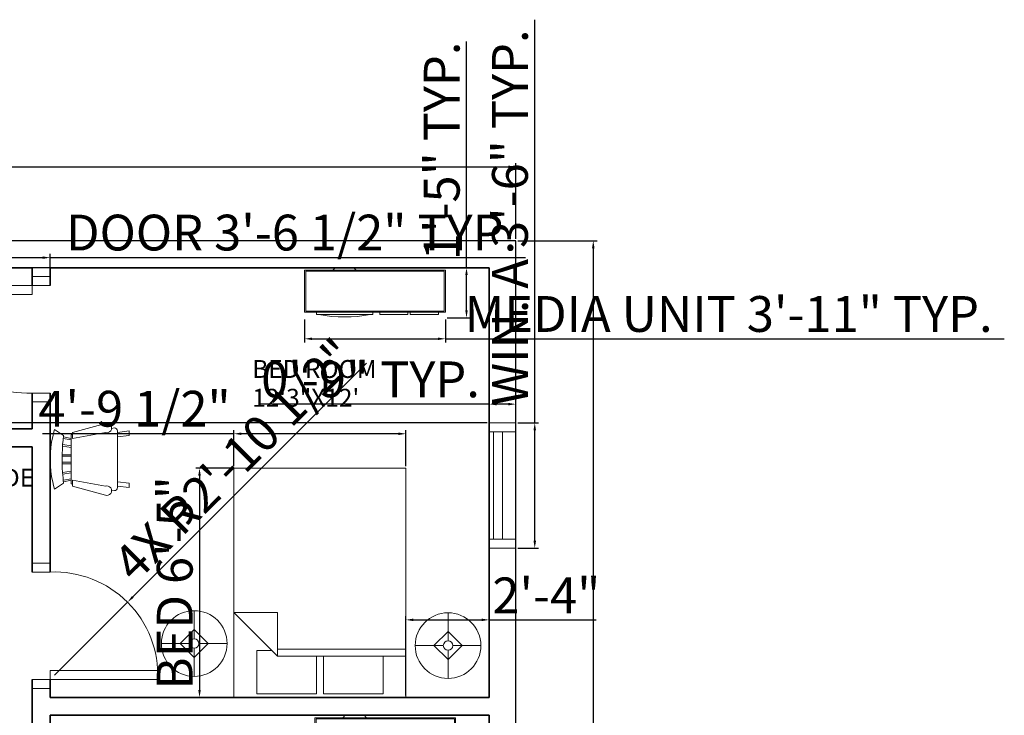
# Model space of a CAD drawing. Units: inches. Extents: x 2021 to 2692, y 429 to 1061.
# Tile 5 of 5: x 2362 to 2692, y 828 to 1061. Entities that reach past the tile are written whole.
import ezdxf

# ---------------------------------------------------------------- set-up
doc = ezdxf.new("R2010")
doc.units = ezdxf.units.IN
for name, color, linetype, lineweight in [('A-ANNO-DIMS', 2, 'Continuous', 18), ('A-AREA-IDEN', 7, 'Continuous', 18), ('A-DOOR', 4, 'Continuous', 18), ('A-FURN', 8, 'Continuous', 13), ('A-GLAZ', 4, 'Continuous', 18), ('A-WALL', 7, 'Continuous', 35), ('C-PROP', 3, 'Continuous', 25)]:
    doc.layers.add(name, color=color, linetype=linetype, lineweight=lineweight)
doc.styles.get("Standard").update_dxf_attribs({"font": 'arial.ttf'})
doc.dimstyles.new('ISO-25', dxfattribs={"dimtxt": 12, "dimasz": 2.5, "dimexe": 1.25, "dimexo": 0.625, "dimtad": 1, "dimdec": 0, "dimlunit": 3, "dimtxsty": 'Standard', "dimcen": 2.5, "dimadec": 0, "dimazin": 0, "dimtfac": 1, "dimtdec": 0, "dimtmove": 0, "dimatfit": 3, "dimfxl": 1, "dimarcsym": 0})

# ---------------------------------------------------------------- blocks, each defined once
blk = doc.blocks.new('Bed - Queen')
for p, q in [((0, -80.00003), (0, 0)), ((0, 0), (59.99999, 0)), ((59.99999, 0), (59.99999, -80.00003)), ((7.99999, -1.2), (28.79998, -1.2)), ((7.99999, -14.4), (7.99999, -1.2)), ((28.79998, -1.2), (28.79998, -14.4)), ((31.19999, -1.2), (51.99999, -1.2)), ((31.19999, -14.4), (31.19999, -1.2)), ((51.99999, -1.2), (51.99999, -16.4)), ((0, -14.4), (44.8, -14.4)), ((44.8, -16.8), (0, -16.8)), ((59.99999, -29.6), (44.8, -14.4)), ((44.8, -14.4), (44.8, -29.6)), ((51.99999, -16.4), (46.79936, -16.4)), ((44.8, -29.6), (59.99999, -29.6)), ((59.99999, -80.00003), (0, -80.00003))]:
    blk.add_line(p, q)
blk = doc.blocks.new('Entertainment Center')
for p, q in [((-4, 0), (-5, -1)), ((4, 0), (-4, 0)), ((5, -1), (4, 0)), ((-17, -19), (-17, -1)), ((-17, -1), (43, -1)), ((-16.5, -18.5), (-16.5, -1.5)), ((-16.5, -1.5), (42.5, -1.5)), ((42.5, -1.5), (42.5, -18.5)), ((43, -1), (43, -19)), ((43, -19), (-17, -19)), ((42.5, -18.5), (-16.5, -18.5)), ((-12, -20), (-12, -19)), ((12, -20), (-12, -20)), ((12, -19), (12, -20)), ((15, -20), (15, -19)), ((27, -20), (15, -20)), ((27, -19), (27, -20)), ((28, -20), (28, -19)), ((40, -20), (28, -20)), ((40, -19), (40, -20))]:
    blk.add_line(p, q)
blk.add_arc((0, 40), 61, 259.6111, 280.3889)
blk = doc.blocks.new('Chair - Rocking')
for p, q in [((-8, -4.5), (-10, -1.5)), ((8, -4.5), (10, -1.5)), ((-7.5, -4.5), (-7, -7)), ((-6.5, -7), (-7.02225, -4.43)), ((-4.5, -7), (-4.96674, -4.19951)), ((-4, -7), (-4.40532, -4.16272)), ((-1.5, -4.05012), (-1.5, -7)), ((-1, -7), (-1, -4.05012)), ((1, -7), (1, -4.04655)), ((1.5, -4.05012), (1.5, -7)), ((4, -7), (4.40187, -4.18694)), ((4.5, -7), (4.96761, -4.19437)), ((6.5, -7), (7, -4.4057)), ((7.5, -4.5), (7, -7)), ((-9, -7.5), (-12, -18.49999)), ((-7, -7.5), (-9, -7.5)), ((-9, -18.49999), (-7, -7.5)), ((-8.23428, -6.99939), (-8.3093, -7.47958)), ((-8.23041, -7), (8.23915, -7)), ((7, -7.5), (9, -7.5)), ((9, -18.49999), (7, -7.5)), ((8.31071, -7.48854), (8.23449, -7.00073)), ((9, -7.5), (12, -18.49999)), ((-10.36644, -20.64523), (-10.5, -21.49999)), ((-9, -22.49999), (-9.5, -26.49999)), ((0, -22.49999), (-9.5, -22.49999)), ((-8, -26.49999), (-7.5, -22.49999)), ((0, -22.49999), (9.5, -22.49999)), ((8, -26.49999), (7.5, -22.49999)), ((9, -22.49999), (9.5, -26.49999)), ((10.5, -21.49999), (10.3575, -20.58798)), ((-9.5, -26.49999), (-8, -26.49999)), ((9.5, -26.49999), (8, -26.49999))]:
    blk.add_line(p, q)
for centre, radius, start, end in [((0, -34.08333), 34.08333, 72.93847, 107.0615), ((0, -68.25004), 64.25, 93.92211, 97.15267), ((0, -68.25004), 64.25, 82.84733, 93.92211), ((-10.5, -18.99999), 1.58114, 161.5651, 18.43495), ((10.5, -18.99999), 1.58114, 161.5651, 18.43495), ((-9.5, -21.49999), 1, 180, 270), ((9.5, -21.49999), 1, 270, 0)]:
    blk.add_arc(centre, radius, start, end)
blk = doc.blocks.new('Lamp - Table')
for p, q in [((0, 7), (0, 1)), ((0, 3), (-3, 0)), ((3, 0), (0, 3)), ((-1, 0), (-7, 0)), ((-3, 0), (0, -3)), ((0, -3), (3, 0)), ((1, 0), (7, 0)), ((0, -1), (0, -7))]:
    blk.add_line(p, q)
for radius in [7, 1]:
    blk.add_circle((0, 0), radius)
blk = doc.blocks.new('*D15')
at = {"layer": 'A-ANNO-DIMS', "color": 0, "lineweight": -2, "transparency": 16777216}
for p, q in [((2168.11, 987.59), (2168.11, 1013.02)), ((2528.11, 987.59), (2528.11, 1013.02)), ((2170.61, 1011.77), (2525.61, 1011.77))]:
    blk.add_line(p, q, dxfattribs=at)
at = {"layer": 'A-ANNO-DIMS', "color": 0, "transparency": 16777216}
for points in [[(2170.61, 1012.18), (2170.61, 1011.35), (2168.11, 1011.77)], [(2525.61, 1012.18), (2525.61, 1011.35), (2528.11, 1011.77)]]:
    blk.add_solid(points, dxfattribs=at)
at = {"layer": 'Defpoints', "color": 0, "transparency": 16777216}
for p in [(2528.11, 1011.77), (2168.11, 986.96), (2528.11, 986.96)]:
    blk.add_point(p, dxfattribs=at)
at = {"layer": 'A-ANNO-DIMS', "color": 0, "transparency": 16777216, "insert": (2348.11, 1018.52), "char_height": 12, "attachment_point": 5}
blk.add_mtext("30'", dxfattribs=at)
blk = doc.blocks.new('*D16')
at = {"layer": 'A-ANNO-DIMS', "color": 0, "lineweight": -2, "transparency": 16777216}
for p, q in [((2528.73, 986.96), (2555.26, 986.96)), ((2554.01, 984.46), (2554.01, 509.46)), ((2528.73, 506.96), (2555.26, 506.96))]:
    blk.add_line(p, q, dxfattribs=at)
at = {"layer": 'A-ANNO-DIMS', "color": 0, "transparency": 16777216}
for points in [[(2553.59, 984.46), (2554.43, 984.46), (2554.01, 986.96)], [(2553.59, 509.46), (2554.43, 509.46), (2554.01, 506.96)]]:
    blk.add_solid(points, dxfattribs=at)
at = {"layer": 'Defpoints', "color": 0, "transparency": 16777216}
for p in [(2528.11, 986.96), (2528.11, 506.96), (2554.01, 506.96)]:
    blk.add_point(p, dxfattribs=at)
at = {"layer": 'A-ANNO-DIMS', "color": 0, "transparency": 16777216, "insert": (2547.26, 746.96), "char_height": 12, "attachment_point": 5, "rotation": 90}
blk.add_mtext("40'", dxfattribs=at)
blk = doc.blocks.new('DOOR-SWING-36IN')
for p, q in [((36.03, 42), (42.03, 42)), ((36.03, 39), (42.03, 39)), ((36.03, 3), (42.03, 3)), ((36.03, 0), (42.03, 0))]:
    blk.add_line(p, q)
blk.add_lwpolyline([(36.03, 39), (0.03, 39), (0.03, 36), (36.03, 36)], close=True)
blk.add_arc((34.53, 37.5), 34.53, 177.5104, 272.4896)
blk = doc.blocks.new('WIN-36IN')
for p, q in [((0, 0), (0, 9)), ((3, 9), (39, 9)), ((3, 0), (3, 9)), ((3, 7.5), (39, 7.5)), ((39, 9), (39, 0)), ((42, 9), (42, 0)), ((3, 4.5), (39, 4.5)), ((39, 0), (3, 0))]:
    blk.add_line(p, q)
blk = doc.blocks.new('*D20')
at = {"layer": 'A-ANNO-DIMS', "color": 0, "lineweight": -2, "transparency": 16777216}
for p, q in [((2329.69, 975.59), (2329.69, 982.58)), ((2332.19, 981.33), (2369.61, 981.33)), ((2372.11, 975.59), (2372.11, 982.58)), ((2372.11, 981.33), (2531.32, 981.33))]:
    blk.add_line(p, q, dxfattribs=at)
at = {"layer": 'A-ANNO-DIMS', "color": 0, "transparency": 16777216}
for points in [[(2332.19, 981.74), (2332.19, 980.91), (2329.69, 981.33)], [(2369.61, 981.74), (2369.61, 980.91), (2372.11, 981.33)]]:
    blk.add_solid(points, dxfattribs=at)
at = {"layer": 'Defpoints', "color": 0, "transparency": 16777216}
for p in [(2372.11, 981.33), (2329.69, 974.96), (2372.11, 974.96)]:
    blk.add_point(p, dxfattribs=at)
at = {"layer": 'A-ANNO-DIMS', "color": 0, "transparency": 16777216, "insert": (2452.96, 988.17), "char_height": 12, "attachment_point": 5}
blk.add_mtext('DOOR 3\'-6 1/2" TYP.', dxfattribs=at)
blk = doc.blocks.new('*D26')
at = {"layer": 'A-ANNO-DIMS', "color": 0, "lineweight": -2, "transparency": 16777216}
for p, q in [((2433.03, 910.79), (2420.88, 910.79)), ((2422.13, 908.29), (2422.13, 836.46)), ((2433.03, 833.96), (2420.88, 833.96))]:
    blk.add_line(p, q, dxfattribs=at)
at = {"layer": 'A-ANNO-DIMS', "color": 0, "transparency": 16777216}
for points in [[(2421.71, 908.29), (2422.55, 908.29), (2422.13, 910.79)], [(2421.71, 836.46), (2422.55, 836.46), (2422.13, 833.96)]]:
    blk.add_solid(points, dxfattribs=at)
at = {"layer": 'Defpoints', "color": 0, "transparency": 16777216}
for p in [(2433.65, 910.79), (2422.13, 833.96), (2433.65, 833.96)]:
    blk.add_point(p, dxfattribs=at)
at = {"layer": 'A-ANNO-DIMS', "color": 0, "transparency": 16777216, "insert": (2415.38, 872.37), "char_height": 12, "attachment_point": 5, "rotation": 90}
blk.add_mtext('BED 6\'-5"', dxfattribs=at)
blk = doc.blocks.new('*D27')
at = {"layer": 'A-ANNO-DIMS', "color": 0, "lineweight": -2, "transparency": 16777216}
for p, q in [((2433.65, 911.41), (2433.65, 923.56)), ((2491.27, 911.41), (2491.27, 923.56)), ((2433.65, 922.31), (2369.56, 922.31)), ((2488.77, 922.31), (2436.15, 922.31))]:
    blk.add_line(p, q, dxfattribs=at)
at = {"layer": 'A-ANNO-DIMS', "color": 0, "transparency": 16777216}
for points in [[(2436.15, 922.73), (2436.15, 921.89), (2433.65, 922.31)], [(2488.77, 922.73), (2488.77, 921.89), (2491.27, 922.31)]]:
    blk.add_solid(points, dxfattribs=at)
at = {"layer": 'Defpoints', "color": 0, "transparency": 16777216}
for p in [(2433.65, 922.31), (2433.65, 910.79), (2491.27, 910.79)]:
    blk.add_point(p, dxfattribs=at)
at = {"layer": 'A-ANNO-DIMS', "color": 0, "transparency": 16777216, "insert": (2400.36, 929.14), "char_height": 12, "attachment_point": 5}
blk.add_mtext('4\'-9 1/2"', dxfattribs=at)
blk = doc.blocks.new('*D30')
at = {"layer": 'A-ANNO-DIMS', "color": 0, "lineweight": -2, "transparency": 16777216}
for p, q in [((2457.34, 960.58), (2457.34, 952.88)), ((2504.48, 960.58), (2504.48, 952.88)), ((2459.84, 954.13), (2501.98, 954.13)), ((2504.48, 954.13), (2691.67, 954.13))]:
    blk.add_line(p, q, dxfattribs=at)
at = {"layer": 'A-ANNO-DIMS', "color": 0, "transparency": 16777216}
for points in [[(2459.84, 954.55), (2459.84, 953.71), (2457.34, 954.13)], [(2501.98, 954.55), (2501.98, 953.71), (2504.48, 954.13)]]:
    blk.add_solid(points, dxfattribs=at)
at = {"layer": 'Defpoints', "color": 0, "transparency": 16777216}
for p in [(2457.34, 961.2), (2504.48, 961.2), (2504.48, 954.13)]:
    blk.add_point(p, dxfattribs=at)
at = {"layer": 'A-ANNO-DIMS', "color": 0, "transparency": 16777216, "insert": (2599.33, 960.89), "char_height": 12, "attachment_point": 5}
blk.add_mtext('MEDIA UNIT 3\'-11" TYP.', dxfattribs=at)
blk = doc.blocks.new('*D31')
at = {"layer": 'A-ANNO-DIMS', "color": 0, "lineweight": -2, "transparency": 16777216}
for p, q in [((2511.56, 977.96), (2511.56, 1053.73)), ((2505.11, 977.96), (2512.81, 977.96)), ((2511.56, 963.7), (2511.56, 975.46)), ((2505.11, 961.2), (2512.81, 961.2))]:
    blk.add_line(p, q, dxfattribs=at)
at = {"layer": 'A-ANNO-DIMS', "color": 0, "transparency": 16777216}
for points in [[(2511.14, 975.46), (2511.97, 975.46), (2511.56, 977.96)], [(2511.14, 963.7), (2511.97, 963.7), (2511.56, 961.2)]]:
    blk.add_solid(points, dxfattribs=at)
at = {"layer": 'Defpoints', "color": 0, "transparency": 16777216}
for p in [(2504.48, 977.96), (2511.56, 977.96), (2504.48, 961.2)]:
    blk.add_point(p, dxfattribs=at)
at = {"layer": 'A-ANNO-DIMS', "color": 0, "transparency": 16777216, "insert": (2504.8, 1017.1), "char_height": 12, "attachment_point": 5, "rotation": 90}
blk.add_mtext('1\'-5" TYP.', dxfattribs=at)
blk = doc.blocks.new('*D32')
at = {"layer": 'A-ANNO-DIMS', "color": 0, "lineweight": -2, "transparency": 16777216}
for p, q in [((2534.41, 925.94), (2534.41, 1061.06)), ((2528.73, 925.94), (2535.66, 925.94)), ((2534.41, 886.44), (2534.41, 923.44)), ((2528.73, 883.94), (2535.66, 883.94))]:
    blk.add_line(p, q, dxfattribs=at)
at = {"layer": 'A-ANNO-DIMS', "color": 0, "transparency": 16777216}
for points in [[(2533.99, 923.44), (2534.83, 923.44), (2534.41, 925.94)], [(2533.99, 886.44), (2534.83, 886.44), (2534.41, 883.94)]]:
    blk.add_solid(points, dxfattribs=at)
at = {"layer": 'Defpoints', "color": 0, "transparency": 16777216}
for p in [(2528.11, 925.94), (2534.41, 925.94), (2528.11, 883.94)]:
    blk.add_point(p, dxfattribs=at)
at = {"layer": 'A-ANNO-DIMS', "color": 0, "transparency": 16777216, "insert": (2527.65, 994.75), "char_height": 12, "attachment_point": 5, "rotation": 90}
blk.add_mtext('WIN. A 3\'-6" TYP.', dxfattribs=at)
blk = doc.blocks.new('*D33')
at = {"layer": 'A-ANNO-DIMS', "color": 0, "lineweight": -2, "transparency": 16777216}
for p, q in [((2519.11, 926.56), (2519.11, 933.49)), ((2528.11, 926.56), (2528.11, 933.49)), ((2519.11, 932.24), (2442.21, 932.24)), ((2525.61, 932.24), (2521.61, 932.24))]:
    blk.add_line(p, q, dxfattribs=at)
at = {"layer": 'A-ANNO-DIMS', "color": 0, "transparency": 16777216}
for points in [[(2521.61, 932.65), (2521.61, 931.82), (2519.11, 932.24)], [(2525.61, 932.65), (2525.61, 931.82), (2528.11, 932.24)]]:
    blk.add_solid(points, dxfattribs=at)
at = {"layer": 'Defpoints', "color": 0, "transparency": 16777216}
for p in [(2519.11, 932.24), (2519.11, 925.94), (2528.11, 925.94)]:
    blk.add_point(p, dxfattribs=at)
at = {"layer": 'A-ANNO-DIMS', "color": 0, "transparency": 16777216, "insert": (2479.41, 938.99), "char_height": 12, "attachment_point": 5}
blk.add_mtext('0\'-9" TYP.', dxfattribs=at)
blk = doc.blocks.new('*D63')
at = {"layer": 'A-ANNO-DIMS', "color": 0, "lineweight": -2, "transparency": 16777216}
for p, q in [((2518.48, 977.96), (2140.87, 977.96)), ((2142.12, 975.46), (2142.12, 928.44)), ((2518.48, 925.94), (2140.87, 925.94))]:
    blk.add_line(p, q, dxfattribs=at)
at = {"layer": 'A-ANNO-DIMS', "color": 0, "transparency": 16777216}
for points in [[(2141.71, 975.46), (2142.54, 975.46), (2142.12, 977.96)], [(2141.71, 928.44), (2142.54, 928.44), (2142.12, 925.94)]]:
    blk.add_solid(points, dxfattribs=at)
at = {"layer": 'Defpoints', "color": 0, "transparency": 16777216}
for p in [(2519.11, 977.96), (2142.12, 925.94), (2519.11, 925.94)]:
    blk.add_point(p, dxfattribs=at)
at = {"layer": 'A-ANNO-DIMS', "color": 0, "transparency": 16777216, "insert": (2135.5, 951.95), "char_height": 12, "attachment_point": 5, "rotation": 90}
blk.add_mtext('4\'-4"', dxfattribs=at)
blk = doc.blocks.new('*D71')
at = {"layer": 'A-ANNO-DIMS', "color": 0, "lineweight": -2, "transparency": 16777216}
for p, q in [((2491.27, 834.59), (2491.27, 861.2)), ((2519.11, 834.59), (2519.11, 861.2)), ((2493.77, 859.95), (2516.61, 859.95)), ((2519.11, 859.95), (2554.96, 859.95))]:
    blk.add_line(p, q, dxfattribs=at)
at = {"layer": 'A-ANNO-DIMS', "color": 0, "transparency": 16777216}
for points in [[(2493.77, 860.37), (2493.77, 859.53), (2491.27, 859.95)], [(2516.61, 860.37), (2516.61, 859.53), (2519.11, 859.95)]]:
    blk.add_solid(points, dxfattribs=at)
at = {"layer": 'Defpoints', "color": 0, "transparency": 16777216}
for p in [(2519.11, 859.95), (2491.27, 833.96), (2519.11, 833.96)]:
    blk.add_point(p, dxfattribs=at)
at = {"layer": 'A-ANNO-DIMS', "color": 0, "transparency": 16777216, "insert": (2538.29, 866.6), "char_height": 12, "attachment_point": 5}
blk.add_mtext('2\'-4"', dxfattribs=at)
blk = doc.blocks.new('*D73')
at = {"layer": 'A-ANNO-DIMS', "color": 0, "lineweight": -2, "transparency": 16777216}
for p, q in [((2478.06, 945.92), (2399.8, 867.65)), ((2373.61, 841.46), (2398.03, 865.88))]:
    blk.add_line(p, q, dxfattribs=at)
at = {"layer": 'A-ANNO-DIMS', "color": 0, "transparency": 16777216}
blk.add_solid([(2399.5, 867.94), (2400.09, 867.36), (2398.03, 865.88)], dxfattribs=at)
at = {"layer": 'Defpoints', "color": 0, "transparency": 16777216}
for p in [(2398.03, 865.88), (2373.61, 841.46)]:
    blk.add_point(p, dxfattribs=at)
at = {"layer": 'A-ANNO-DIMS', "color": 0, "transparency": 16777216, "insert": (2434.98, 912.5), "char_height": 12, "attachment_point": 5, "rotation": 44.9994}
blk.add_mtext('4X R2\'-10 1/2"', dxfattribs=at)

msp = doc.modelspace()

# ---------------------------------------------------------------- linework, layer by layer
at = {"layer": 'A-WALL'}
for p, q in [((2366.11, 977.96), (2270.11, 977.96)), ((2366.11, 971.96), (2366.11, 977.96)), ((2519.11, 977.96), (2372.11, 977.96)), ((2372.11, 971.96), (2372.11, 977.96)), ((2519.11, 833.96), (2519.11, 977.96)), ((2366.11, 923.96), (2366.11, 935.96)), ((2372.11, 875.96), (2372.11, 935.96)), ((2366.11, 923.96), (2270.11, 923.96)), ((2366.11, 917.96), (2330.11, 917.96)), ((2366.11, 875.96), (2366.11, 917.96)), ((2366.11, 833.96), (2366.11, 839.96)), ((2372.11, 833.96), (2372.11, 839.96)), ((2366.11, 833.96), (2366.11, 827.96)), ((2519.11, 833.96), (2372.11, 833.96)), ((2366.11, 821.96), (2366.11, 827.96)), ((2519.11, 827.96), (2372.11, 827.96)), ((2372.11, 821.96), (2372.11, 827.96)), ((2519.11, 707.96), (2519.11, 827.96))]:
    msp.add_line(p, q, dxfattribs=at)
at = {"layer": 'C-PROP'}
msp.add_lwpolyline([(2168.11, 506.96), (2528.11, 506.96), (2528.11, 986.96), (2168.11, 986.96)], close=True, dxfattribs=at)

# ---------------------------------------------------------------- block references
at = {"layer": 'A-DOOR'}
msp.add_blockref('DOOR-SWING-36IN', (2330.08, 932.96), dxfattribs=at)
at = {"layer": 'A-DOOR', "rotation": 180}
msp.add_blockref('DOOR-SWING-36IN', (2408.14, 878.96), dxfattribs=at)
at = {"layer": 'A-FURN'}
for name, p, xscale, yscale, zscale in [('Entertainment Center', (2470.7, 977.96), 0.7857640072773148, 0.7857640072773148, 0.7857640072773148), ('Lamp - Table', (2420.36, 852.02), 1.571428663265289, 1.571428663265289, 1.571428663265289), ('Lamp - Table', (2505.36, 851.33), 1.571428663265289, 1.571428663265289, 1.571428663265289), ('Entertainment Center', (2474.11, 827.96), 0.7857640072773148, 0.7857640072773148, 0.7857640072773148)]:
    msp.add_blockref(name, p, dxfattribs=dict(at, xscale=xscale, yscale=yscale, zscale=zscale))
at = {"layer": 'A-FURN', "rotation": 90}
msp.add_blockref('Chair - Rocking', (2372.11, 913.75), dxfattribs=at)
at = {"layer": 'A-FURN', "xscale": 0.9602656441849337, "yscale": 0.9602656441849337, "zscale": 0.9602656441849337, "rotation": 180}
msp.add_blockref('Bed - Queen', (2491.27, 833.96), dxfattribs=at)
at = {"layer": 'A-GLAZ', "rotation": 89.999999999998}
msp.add_blockref('WIN-36IN', (2528.11, 883.94), dxfattribs=at)

# ---------------------------------------------------------------- texts
at = {"layer": 'A-AREA-IDEN'}
for s, p in [('BED ROOM', (2439.79, 941.01)), ('12\'3"X12\'', (2439.79, 931.37)), ('3\'2"WIDE', (2331.45, 904.59))]:
    msp.add_text(s, height=6, dxfattribs=at).set_placement(p)

# ---------------------------------------------------------------- dimensions: what is measured, and where the dimension line sits
at = {"layer": 'A-ANNO-DIMS'}
for base, p1, p2, angle, text, picture, middle in [((2534.41, 925.94), (2528.11, 883.94), (2528.11, 925.94), 90, 'WIN. A <> TYP.', '*D32', (2527.65, 994.75)), ((2511.56, 977.96), (2504.48, 961.2), (2504.48, 977.96), 90, '<> TYP.', '*D31', (2504.8, 1017.1)), ((2519.11, 932.24), (2528.11, 925.94), (2519.11, 925.94), 180, '<> TYP.', '*D33', (2479.41, 938.99)), ((2422.13, 833.96), (2433.65, 910.79), (2433.65, 833.96), 270, 'BED <>', '*D26', (2415.38, 872.37))]:
    dim = msp.add_linear_dim(base=base, p1=p1, p2=p2, angle=angle, text=text, dimstyle='ISO-25', override={"dimdec": 1, "dimlfac": 1, "dimrnd": 0, "dimzin": 1, "dimdsep": 46, "dimlunit": 4, "dimfrac": 2}, dxfattribs=at)
    dim.commit()
    dim.dimension.update_dxf_attribs({"geometry": picture, "text_midpoint": middle})
for base, p1, p2, override, picture, middle in [((2528.11, 1011.77), (2168.11, 986.96), (2528.11, 986.96), {"dimclrd": 0, "dimclre": 0, "dimclrt": 0}, '*D15', (2348.11, 1018.52)), ((2519.11, 859.95), (2491.27, 833.96), (2519.11, 833.96), {"dimdec": 1, "dimlfac": 1, "dimrnd": 0, "dimzin": 1, "dimdsep": 46, "dimlunit": 4, "dimfrac": 2}, '*D71', (2538.29, 866.6))]:
    dim = msp.add_linear_dim(base=base, p1=p1, p2=p2, dimstyle='ISO-25', override=override, dxfattribs=at)
    dim.commit()
    dim.dimension.update_dxf_attribs({"geometry": picture, "text_midpoint": middle})
for base, p1, p2, text, picture, middle in [((2372.11, 981.33), (2329.69, 974.96), (2372.11, 974.96), 'DOOR <> TYP.', '*D20', (2452.96, 988.17)), ((2504.48, 954.13), (2457.34, 961.2), (2504.48, 961.2), 'MEDIA UNIT <> TYP.', '*D30', (2599.33, 960.89))]:
    dim = msp.add_linear_dim(base=base, p1=p1, p2=p2, text=text, dimstyle='ISO-25', override={"dimdec": 1, "dimlfac": 1, "dimrnd": 0, "dimzin": 1, "dimdsep": 46, "dimlunit": 4, "dimfrac": 2}, dxfattribs=at)
    dim.commit()
    dim.dimension.update_dxf_attribs({"geometry": picture, "text_midpoint": middle})
for base, p1, p2, angle, override, picture, middle in [((2554.01, 506.96), (2528.11, 986.96), (2528.11, 506.96), 90, {"dimclrd": 0, "dimclre": 0, "dimclrt": 0}, '*D16', (2547.26, 746.96)), ((2142.12, 925.94), (2519.11, 977.96), (2519.11, 925.94), 90, {"dimdec": 1, "dimlfac": 1, "dimrnd": 0, "dimzin": 1, "dimdsep": 46, "dimlunit": 4, "dimfrac": 2}, '*D63', (2135.5, 951.95)), ((2433.65, 922.31), (2491.27, 910.79), (2433.65, 910.79), 180, {"dimdec": 1, "dimlfac": 1, "dimrnd": 0, "dimzin": 1, "dimdsep": 46, "dimlunit": 4, "dimfrac": 2}, '*D27', (2400.36, 929.14))]:
    dim = msp.add_linear_dim(base=base, p1=p1, p2=p2, angle=angle, dimstyle='ISO-25', override=override, dxfattribs=at)
    dim.commit()
    dim.dimension.update_dxf_attribs({"geometry": picture, "text_midpoint": middle})
dim = msp.add_radius_dim(center=(2373.61, 841.46), mpoint=(2398.03, 865.88), text='4X <>', dimstyle='ISO-25', override={"dimdec": 1, "dimlfac": 1, "dimrnd": 0, "dimzin": 1, "dimdsep": 46, "dimlunit": 4, "dimfrac": 2}, dxfattribs=at)
dim.commit()
dim.dimension.update_dxf_attribs({"geometry": '*D73', "text_midpoint": (2434.98, 912.5)})

doc.saveas('drawing.dxf')
